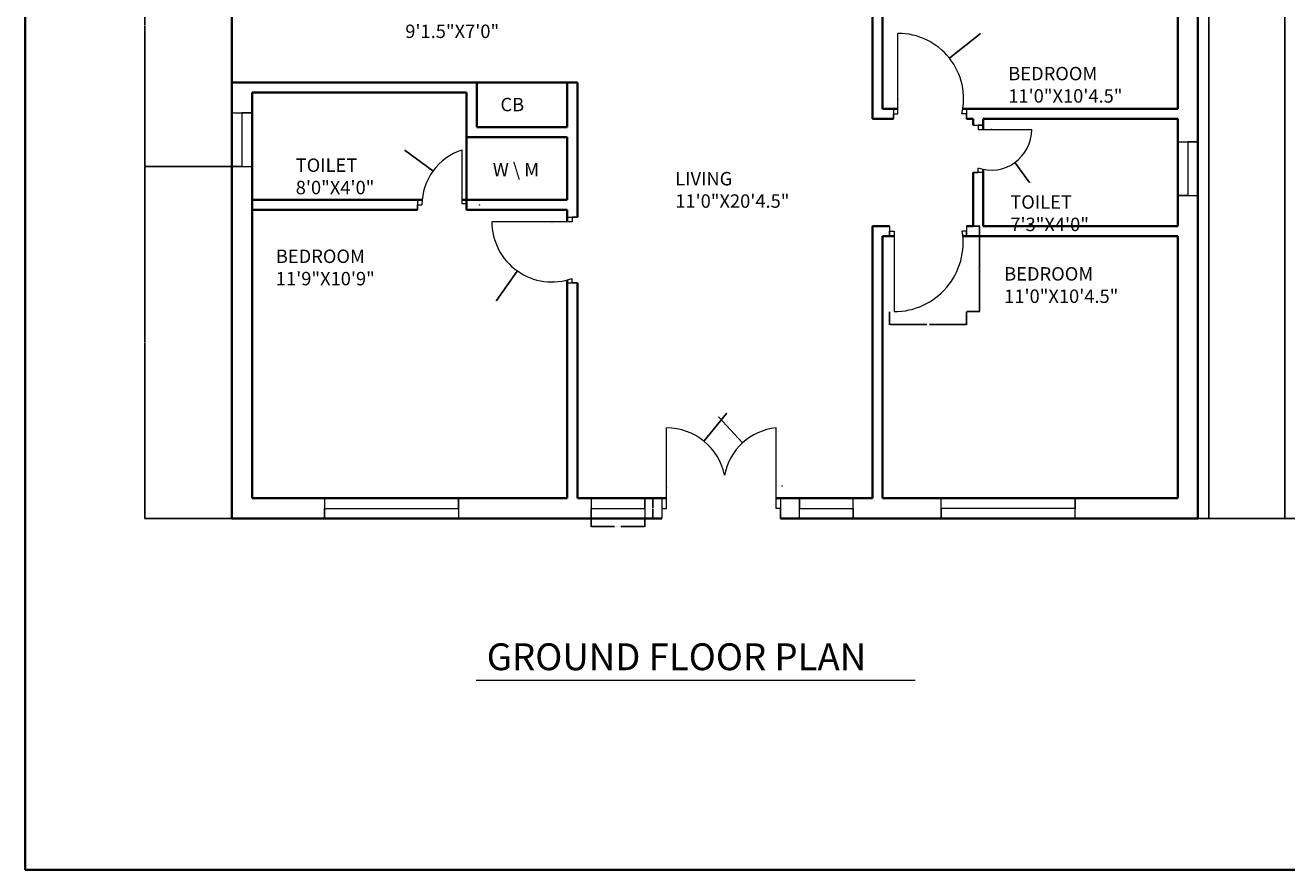
# Model space of a CAD drawing. Units: inches. Extents: x 2250 to 3547, y 1387 to 2604.
# Tile 1 of 11: x 2250 to 2814, y 1387 to 1765. Entities that reach past the tile are written whole.
import ezdxf

# ---------------------------------------------------------------- set-up
doc = ezdxf.new("R2010")
doc.units = ezdxf.units.IN
for name, color, linetype, lineweight in [('A-ANNO-DIMS', 2, 'Continuous', 18), ('A-ANNO-TEXT', 7, 'Continuous', 18), ('A-ANNO-TTLB', 7, 'Continuous', 35), ('A-AREA-IDEN', 7, 'Continuous', 18), ('A-DOOR', 3, 'Continuous', 18), ('A-GLAZ', 4, 'Continuous', 18), ('A-WALL', 7, 'Continuous', 35)]:
    doc.layers.add(name, color=color, linetype=linetype, lineweight=lineweight)
doc.styles.get("Standard").update_dxf_attribs({"font": 'arial.ttf'})
doc.dimstyles.get("Standard").update_dxf_attribs({"dimtxt": 0.18, "dimasz": 0.18, "dimexe": 0.18, "dimexo": 0.0625, "dimgap": 0.09, "dimtad": 0, "dimtih": 1, "dimtoh": 1, "dimdec": 4, "dimzin": 0, "dimdsep": 46, "dimtxsty": 'Standard', "dimcen": 0.09, "dimadec": 0, "dimazin": 0, "dimtfac": 1, "dimtdec": 4, "dimtofl": 0, "dimtmove": 0, "dimatfit": 3, "dimfxl": 1, "dimtolj": 1, "dimtzin": 0, "dimarcsym": 0})

# ---------------------------------------------------------------- blocks, each defined once
blk = doc.blocks.new('WIN-24')
for p, q in [((0, 24), (9, 24)), ((9, 24), (4.5, 24)), ((4.5, 24), (4.5, 0)), ((4.5, 0), (0, 0)), ((0, 0), (9, 0))]:
    blk.add_line(p, q)
blk = doc.blocks.new('WIN-60')
for p, q in [((0, 9), (0, 0)), ((60, 4.5), (60, 9)), ((60, 9), (60, 0)), ((0, 0), (0, 4.5)), ((0, 4.5), (60, 4.5))]:
    blk.add_line(p, q)
blk = doc.blocks.new('WIN-24-SPLIT')
for p, q in [((0, 9), (0, 0)), ((24, 4.5), (24, 9)), ((24, 9), (24, 0)), ((0, 0), (0, 4.5)), ((0, 4.5), (12, 4.5)), ((12, 4.5), (24, 4.5))]:
    blk.add_line(p, q)
blk = doc.blocks.new('DOOR-ENTRY-DOUBLE-SOUTH')
for p, q in [((2, 4.5), (2, 40.5)), ((51.02, 4.5), (51.02, 40.5)), ((0, 9), (0, 0)), ((53.02, 9), (53.02, 0)), ((0, 4.5), (2, 4.5)), ((53.02, 4.5), (51.02, 4.5)), ((53.02, 0), (53.02, 4.5))]:
    blk.add_line(p, q)
for centre, radius, start, end in [((2, 13.91), 26.59, 11.9677, 90), ((53.68, 14.51), 26.13, 95.8256, 169.162)]:
    blk.add_arc(centre, radius, start, end)
blk = doc.blocks.new('DOOR-BED-SOUTHEAST')
for p, q in [((0, 38.25), (0, 33.75)), ((0, 33.75), (0, 36)), ((0, 36), (2, 36)), ((2, 36), (2, 0)), ((34.44, 36), (32.44, 36)), ((34.44, 38.25), (34.44, 33.75)), ((34.44, 33.75), (34.44, 36))]:
    blk.add_line(p, q)
blk.add_arc((2, 30.87), 30.87, 270, 9.5589)
blk = doc.blocks.new('DOOR-BED-WEST-S')
for p, q in [((33.75, 29.39), (38.25, 29.39)), ((38.25, 29.39), (36, 29.39)), ((36, 29.39), (36, 27.39)), ((36, 27.39), (0, 27.39)), ((36, 0), (36, 2)), ((33.75, 0), (38.25, 0)), ((38.25, 0), (36, 0))]:
    blk.add_line(p, q)
blk.add_arc((26.95, 27.39), 26.95, 180, 289.6121)
blk = doc.blocks.new('DOOR-BED-EAST-S')
for p, q in [((2, 2.25), (2, 38.25)), ((0, 4.5), (0, 0)), ((0, 0), (0, 2.25)), ((0, 2.25), (2, 2.25)), ((32.6, 2.25), (30.6, 2.25)), ((32.6, 4.5), (32.6, 0)), ((32.6, 0), (32.6, 2.25))]:
    blk.add_line(p, q)
blk.add_arc((2, 8.89), 29.36, 346.921, 90)
blk = doc.blocks.new('DOOR-BATH-EAST-S')
for p, q in [((0, 21.23), (4.5, 21.23)), ((4.5, 21.23), (2.25, 21.23)), ((2.25, 21.23), (2.25, 19.23)), ((2.25, 19.23), (26.25, 19.23)), ((4.5, 0), (0, 0)), ((0, 0), (2.25, 0)), ((2.25, 0), (2.25, 2))]:
    blk.add_line(p, q)
blk.add_arc((8.07, 19.23), 18.18, 251.336, 0)
blk = doc.blocks.new('DOOR-BATH-WEST-S')
for p, q in [((19.98, 2.81), (19.98, 26.81)), ((0, 4.5), (0, 0)), ((0, 0), (0, 2.25)), ((0, 2.25), (2, 2.25)), ((21.98, 2.81), (19.98, 2.81)), ((21.98, 0), (21.98, 2.81))]:
    blk.add_line(p, q)
blk.add_arc((27.76, 2.25), 25.76, 107.5855, 180)
blk = doc.blocks.new('*D34')
at = {"layer": 'A-ANNO-DIMS', "color": 0, "lineweight": -2, "transparency": 16777216}
for p, q in [((2503.17, 1543.86), (2503.17, 1540.14)), ((2503.35, 1540.32), (2513.67, 1540.32)), ((2526.99, 1540.32), (2516.67, 1540.32)), ((2527.17, 1543.86), (2527.17, 1540.14))]:
    blk.add_line(p, q, dxfattribs=at)
at = {"layer": 'A-ANNO-DIMS', "color": 0, "transparency": 16777216}
for points in [[(2503.35, 1540.35), (2503.35, 1540.29), (2503.17, 1540.32)], [(2526.99, 1540.35), (2526.99, 1540.29), (2527.17, 1540.32)]]:
    blk.add_solid(points, dxfattribs=at)
at = {"layer": 'Defpoints', "color": 0, "transparency": 16777216}
for p in [(2503.17, 1543.92), (2527.17, 1543.92), (2527.17, 1540.32)]:
    blk.add_point(p, dxfattribs=at)
at = {"layer": 'A-ANNO-DIMS', "color": 0, "transparency": 16777216, "insert": (2515.17, 1540.32), "char_height": 0.18, "attachment_point": 5}
blk.add_mtext('\\A1;SPLIT WINDOW 24 TYP.', dxfattribs=at)
blk = doc.blocks.new('*D35')
at = {"layer": 'A-ANNO-DIMS', "color": 0, "lineweight": -2, "transparency": 16777216}
for p, q in [((2527.23, 1552.92), (2530.95, 1552.92)), ((2530.77, 1552.74), (2530.77, 1548.61)), ((2530.77, 1544.1), (2530.77, 1548.24)), ((2527.23, 1543.92), (2530.95, 1543.92))]:
    blk.add_line(p, q, dxfattribs=at)
at = {"layer": 'A-ANNO-DIMS', "color": 0, "transparency": 16777216}
for points in [[(2530.74, 1552.74), (2530.8, 1552.74), (2530.77, 1552.92)], [(2530.74, 1544.1), (2530.8, 1544.1), (2530.77, 1543.92)]]:
    blk.add_solid(points, dxfattribs=at)
at = {"layer": 'Defpoints', "color": 0, "transparency": 16777216}
for p in [(2527.17, 1552.92), (2530.77, 1552.92), (2527.17, 1543.92)]:
    blk.add_point(p, dxfattribs=at)
at = {"layer": 'A-ANNO-DIMS', "color": 0, "transparency": 16777216, "insert": (2530.77, 1548.42), "char_height": 0.18, "attachment_point": 5}
blk.add_mtext('\\A1;9 TYP.', dxfattribs=at)
blk = doc.blocks.new('*D46')
at = {"layer": 'A-ANNO-DIMS', "color": 0, "lineweight": -2, "transparency": 16777216}
for p, q in [((2671.22, 1674.7), (2677.08, 1674.7)), ((2676.9, 1674.52), (2676.9, 1655.75)), ((2676.9, 1636.63), (2676.9, 1655.39)), ((2671.22, 1636.45), (2677.08, 1636.45))]:
    blk.add_line(p, q, dxfattribs=at)
at = {"layer": 'A-ANNO-DIMS', "color": 0, "transparency": 16777216}
for points in [[(2676.87, 1674.52), (2676.93, 1674.52), (2676.9, 1674.7)], [(2676.87, 1636.63), (2676.93, 1636.63), (2676.9, 1636.45)]]:
    blk.add_solid(points, dxfattribs=at)
at = {"layer": 'Defpoints', "color": 0, "transparency": 16777216}
for p in [(2671.16, 1674.7), (2676.9, 1674.7), (2671.16, 1636.45)]:
    blk.add_point(p, dxfattribs=at)
at = {"layer": 'A-ANNO-DIMS', "color": 0, "transparency": 16777216, "insert": (2676.9, 1655.57), "char_height": 0.18, "attachment_point": 5}
blk.add_mtext('\\A1;DOOR 38 TYP.', dxfattribs=at)
blk = doc.blocks.new('*D47')
at = {"layer": 'A-ANNO-DIMS', "color": 0, "lineweight": -2, "transparency": 16777216}
for p, q in [((2636.72, 1636.38), (2636.72, 1630.53)), ((2671.16, 1636.38), (2671.16, 1630.53)), ((2636.9, 1630.71), (2653.41, 1630.71)), ((2670.98, 1630.71), (2654.47, 1630.71))]:
    blk.add_line(p, q, dxfattribs=at)
at = {"layer": 'A-ANNO-DIMS', "color": 0, "transparency": 16777216}
for points in [[(2636.9, 1630.74), (2636.9, 1630.68), (2636.72, 1630.71)], [(2670.98, 1630.74), (2670.98, 1630.68), (2671.16, 1630.71)]]:
    blk.add_solid(points, dxfattribs=at)
at = {"layer": 'Defpoints', "color": 0, "transparency": 16777216}
for p in [(2636.72, 1636.45), (2671.16, 1636.45), (2671.16, 1630.71)]:
    blk.add_point(p, dxfattribs=at)
at = {"layer": 'A-ANNO-DIMS', "color": 0, "transparency": 16777216, "insert": (2653.94, 1630.71), "char_height": 0.18, "attachment_point": 5}
blk.add_mtext('\\A1;34 TYP.', dxfattribs=at)
blk = doc.blocks.new('*D77')
at = {"layer": 'A-ANNO-DIMS', "color": 0, "lineweight": -2, "transparency": 16777216}
for p, q in [((2633.6, 2245.18), (2813.67, 2245.18)), ((2813.49, 2245), (2813.49, 1894.73)), ((2813.49, 1544.1), (2813.49, 1894.37)), ((2774.6, 1543.92), (2813.67, 1543.92))]:
    blk.add_line(p, q, dxfattribs=at)
at = {"layer": 'A-ANNO-DIMS', "color": 0, "transparency": 16777216}
for points in [[(2813.46, 2245), (2813.52, 2245), (2813.49, 2245.18)], [(2813.46, 1544.1), (2813.52, 1544.1), (2813.49, 1543.92)]]:
    blk.add_solid(points, dxfattribs=at)
at = {"layer": 'Defpoints', "color": 0, "transparency": 16777216}
for p in [(2633.54, 2245.18), (2813.49, 2245.18), (2774.54, 1543.92)]:
    blk.add_point(p, dxfattribs=at)
at = {"layer": 'A-ANNO-DIMS', "color": 0, "transparency": 16777216, "insert": (2813.49, 1894.55), "char_height": 0.18, "attachment_point": 5}
blk.add_mtext('\\A1;701.3', dxfattribs=at)
blk = doc.blocks.new('*D78')
at = {"layer": 'A-ANNO-DIMS', "color": 0, "lineweight": -2, "transparency": 16777216}
for p, q in [((2342.48, 1701.32), (2303.41, 1701.32)), ((2303.59, 1701.14), (2303.59, 1622.8)), ((2303.59, 1544.1), (2303.59, 1622.44)), ((2342.48, 1543.92), (2303.41, 1543.92))]:
    blk.add_line(p, q, dxfattribs=at)
at = {"layer": 'A-ANNO-DIMS', "color": 0, "transparency": 16777216}
for points in [[(2303.56, 1701.14), (2303.62, 1701.14), (2303.59, 1701.32)], [(2303.56, 1544.1), (2303.62, 1544.1), (2303.59, 1543.92)]]:
    blk.add_solid(points, dxfattribs=at)
at = {"layer": 'Defpoints', "color": 0, "transparency": 16777216}
for p in [(2303.59, 1701.32), (2342.54, 1701.32), (2342.54, 1543.92)]:
    blk.add_point(p, dxfattribs=at)
at = {"layer": 'A-ANNO-DIMS', "color": 0, "transparency": 16777216, "insert": (2303.59, 1622.62), "char_height": 0.18, "attachment_point": 5}
blk.add_mtext('\\A1;157.4', dxfattribs=at)
blk = doc.blocks.new('*D79')
at = {"layer": 'A-ANNO-DIMS', "color": 0, "lineweight": -2, "transparency": 16777216}
for p, q in [((2342.48, 1827.42), (2303.41, 1827.42)), ((2303.59, 1827.24), (2303.59, 1764.55)), ((2303.59, 1701.5), (2303.59, 1764.19)), ((2342.48, 1701.32), (2303.41, 1701.32))]:
    blk.add_line(p, q, dxfattribs=at)
at = {"layer": 'A-ANNO-DIMS', "color": 0, "transparency": 16777216}
for points in [[(2303.56, 1827.24), (2303.62, 1827.24), (2303.59, 1827.42)], [(2303.56, 1701.5), (2303.62, 1701.5), (2303.59, 1701.32)]]:
    blk.add_solid(points, dxfattribs=at)
at = {"layer": 'Defpoints', "color": 0, "transparency": 16777216}
for p in [(2303.59, 1827.42), (2342.54, 1827.42), (2342.54, 1701.32)]:
    blk.add_point(p, dxfattribs=at)
at = {"layer": 'A-ANNO-DIMS', "color": 0, "transparency": 16777216, "insert": (2303.59, 1764.37), "char_height": 0.18, "attachment_point": 5}
blk.add_mtext('\\A1;126.1', dxfattribs=at)
blk = doc.blocks.new('*D85')
at = {"layer": 'A-ANNO-DIMS', "color": 0, "lineweight": -2, "transparency": 16777216}
for p, q in [((3001.57, 2245.18), (2779.34, 2245.18)), ((2779.52, 2245), (2779.52, 1894.73)), ((2779.52, 1544.1), (2779.52, 1894.37)), ((2851.57, 1543.92), (2779.34, 1543.92))]:
    blk.add_line(p, q, dxfattribs=at)
at = {"layer": 'A-ANNO-DIMS', "color": 0, "transparency": 16777216}
for points in [[(2779.49, 2245), (2779.55, 2245), (2779.52, 2245.18)], [(2779.49, 1544.1), (2779.55, 1544.1), (2779.52, 1543.92)]]:
    blk.add_solid(points, dxfattribs=at)
at = {"layer": 'Defpoints', "color": 0, "transparency": 16777216}
for p in [(2779.52, 2245.18), (3001.63, 2245.18), (2851.63, 1543.92)]:
    blk.add_point(p, dxfattribs=at)
at = {"layer": 'A-ANNO-DIMS', "color": 0, "transparency": 16777216, "insert": (2779.52, 1894.55), "char_height": 0.18, "attachment_point": 5}
blk.add_mtext('\\A1;701.3', dxfattribs=at)
blk = doc.blocks.new('*D118')
at = {"layer": 'A-ANNO-DIMS', "color": 0, "lineweight": -2, "transparency": 16777216}
for p, q in [((2677.22, 1760.8), (2663.57, 1749.96)), ((2677.4, 1760.8), (2677.22, 1760.8)), ((2640.35, 1731.59), (2640.53, 1731.59)), ((2640.44, 1731.5), (2640.44, 1731.68))]:
    blk.add_line(p, q, dxfattribs=at)
at = {"layer": 'A-ANNO-DIMS', "color": 0, "transparency": 16777216}
blk.add_solid([(2663.55, 1749.98), (2663.59, 1749.94), (2663.43, 1749.85)], dxfattribs=at)
at = {"layer": 'Defpoints', "color": 0, "transparency": 16777216}
for p in [(2663.43, 1749.85), (2640.44, 1731.59)]:
    blk.add_point(p, dxfattribs=at)
at = {"layer": 'A-ANNO-DIMS', "color": 0, "transparency": 16777216, "insert": (2677.95, 1760.8), "char_height": 0.18, "attachment_point": 5}
blk.add_mtext('\\A1;R29.357', dxfattribs=at)
blk = doc.blocks.new('*D120')
at = {"layer": 'A-ANNO-DIMS', "color": 0, "lineweight": -2, "transparency": 16777216}
for p, q in [((2485.65, 1676.67), (2485.83, 1676.67)), ((2485.74, 1676.58), (2485.74, 1676.76)), ((2460.89, 1641.43), (2470.1, 1654.5)), ((2460.71, 1641.43), (2460.89, 1641.43))]:
    blk.add_line(p, q, dxfattribs=at)
at = {"layer": 'A-ANNO-DIMS', "color": 0, "transparency": 16777216}
blk.add_solid([(2470.08, 1654.51), (2470.13, 1654.48), (2470.21, 1654.64)], dxfattribs=at)
at = {"layer": 'Defpoints', "color": 0, "transparency": 16777216}
for p in [(2485.74, 1676.67), (2470.21, 1654.64)]:
    blk.add_point(p, dxfattribs=at)
at = {"layer": 'A-ANNO-DIMS', "color": 0, "transparency": 16777216, "insert": (2460.16, 1641.43), "char_height": 0.18, "attachment_point": 5}
blk.add_mtext('\\A1;R26.953', dxfattribs=at)
blk = doc.blocks.new('*D121')
at = {"layer": 'A-ANNO-DIMS', "color": 0, "lineweight": -2, "transparency": 16777216}
for p, q in [((2563.69, 1590.89), (2553.76, 1578.63)), ((2563.87, 1590.89), (2563.69, 1590.89)), ((2536.81, 1557.83), (2536.99, 1557.83)), ((2536.9, 1557.74), (2536.9, 1557.92))]:
    blk.add_line(p, q, dxfattribs=at)
at = {"layer": 'A-ANNO-DIMS', "color": 0, "transparency": 16777216}
blk.add_solid([(2553.73, 1578.65), (2553.78, 1578.61), (2553.64, 1578.49)], dxfattribs=at)
at = {"layer": 'Defpoints', "color": 0, "transparency": 16777216}
for p in [(2553.64, 1578.49), (2536.9, 1557.83)]:
    blk.add_point(p, dxfattribs=at)
at = {"layer": 'A-ANNO-DIMS', "color": 0, "transparency": 16777216, "insert": (2564.42, 1590.89), "char_height": 0.18, "attachment_point": 5}
blk.add_mtext('\\A1;R26.593', dxfattribs=at)
blk = doc.blocks.new('*D123')
at = {"layer": 'A-ANNO-DIMS', "color": 0, "lineweight": -2, "transparency": 16777216}
for p, q in [((2560.16, 1589.26), (2560.34, 1589.26)), ((2560.34, 1589.26), (2570.81, 1577.83)), ((2588.49, 1558.43), (2588.67, 1558.43)), ((2588.58, 1558.34), (2588.58, 1558.52))]:
    blk.add_line(p, q, dxfattribs=at)
at = {"layer": 'A-ANNO-DIMS', "color": 0, "transparency": 16777216}
blk.add_solid([(2570.83, 1577.85), (2570.78, 1577.81), (2570.93, 1577.7)], dxfattribs=at)
at = {"layer": 'Defpoints', "color": 0, "transparency": 16777216}
for p in [(2570.93, 1577.7), (2588.58, 1558.43)]:
    blk.add_point(p, dxfattribs=at)
at = {"layer": 'A-ANNO-DIMS', "color": 0, "transparency": 16777216, "insert": (2559.61, 1589.26), "char_height": 0.18, "attachment_point": 5}
blk.add_mtext('\\A1;R26.126', dxfattribs=at)
blk = doc.blocks.new('*D124')
at = {"layer": 'A-ANNO-DIMS', "color": 0, "lineweight": -2, "transparency": 16777216}
for p, q in [((2419.88, 1708.52), (2420.06, 1708.52)), ((2420.06, 1708.52), (2432.39, 1699.5)), ((2453.23, 1684.17), (2453.41, 1684.17)), ((2453.32, 1684.08), (2453.32, 1684.26))]:
    blk.add_line(p, q, dxfattribs=at)
at = {"layer": 'A-ANNO-DIMS', "color": 0, "transparency": 16777216}
blk.add_solid([(2432.41, 1699.52), (2432.37, 1699.48), (2432.53, 1699.39)], dxfattribs=at)
at = {"layer": 'Defpoints', "color": 0, "transparency": 16777216}
for p in [(2432.53, 1699.39), (2453.32, 1684.17)]:
    blk.add_point(p, dxfattribs=at)
at = {"layer": 'A-ANNO-DIMS', "color": 0, "transparency": 16777216, "insert": (2419.4, 1708.52), "char_height": 0.18, "attachment_point": 5}
blk.add_mtext('\\A1;R25.76', dxfattribs=at)
blk = doc.blocks.new('*D128')
at = {"layer": 'A-ANNO-DIMS', "color": 0, "lineweight": -2, "transparency": 16777216}
for p, q in [((2682.02, 1717.92), (2682.2, 1717.92)), ((2682.11, 1717.83), (2682.11, 1718.01)), ((2699.07, 1694.29), (2692.81, 1703.01)), ((2699.25, 1694.29), (2699.07, 1694.29))]:
    blk.add_line(p, q, dxfattribs=at)
at = {"layer": 'A-ANNO-DIMS', "color": 0, "transparency": 16777216}
blk.add_solid([(2692.84, 1703.02), (2692.79, 1702.99), (2692.71, 1703.15)], dxfattribs=at)
at = {"layer": 'Defpoints', "color": 0, "transparency": 16777216}
for p in [(2682.11, 1717.92), (2692.71, 1703.15)]:
    blk.add_point(p, dxfattribs=at)
at = {"layer": 'A-ANNO-DIMS', "color": 0, "transparency": 16777216, "insert": (2699.73, 1694.29), "char_height": 0.18, "attachment_point": 5}
blk.add_mtext('\\A1;R18.18', dxfattribs=at)

msp = doc.modelspace()

# ---------------------------------------------------------------- linework, layer by layer
at = {"layer": 'A-ANNO-TEXT'}
msp.add_line((2451.7239, 1471.575), (2648.1293, 1471.575), dxfattribs=at)
at = {"layer": 'A-ANNO-TTLB'}
msp.add_lwpolyline([(2250.1093, 2604.1988), (3546.995, 2604.1988), (3546.995, 1386.7251), (2250.1093, 1386.7251)], close=True, dxfattribs=at)
at = {"layer": 'A-WALL'}
for p, q in [((2774.5378, 2232.5639), (2774.5378, 1543.9245)), ((2765.5378, 2037.5639), (2765.5378, 1727.1967)), ((2633.5378, 1856.1967), (2633.5378, 1727.1967)), ((2342.5378, 1827.4245), (2342.5378, 1543.9245)), ((2342.5378, 1827.4245), (2342.5378, 1543.9245)), ((2629.0378, 1818.5639), (2629.0378, 1722.6967)), ((2342.5378, 1738.9245), (2492.5378, 1738.9245)), ((2452.0378, 1719.0224), (2452.0378, 1738.9245)), ((2492.5378, 1738.9245), (2497.0378, 1738.9245)), ((2492.5378, 1738.9245), (2492.5378, 1719.0224)), ((2497.0378, 1738.9245), (2497.0378, 1678.669)), ((2351.5378, 1734.4245), (2447.5378, 1734.4245)), ((2351.5378, 1734.4245), (2351.5378, 1552.9245)), ((2351.5378, 1734.4245), (2351.5378, 1686.4245)), ((2351.5378, 1734.4245), (2447.5378, 1734.4245)), ((2447.5378, 1734.4245), (2447.5378, 1714.5224)), ((2640.439, 1727.1967), (2633.5378, 1727.1967)), ((2765.5378, 1727.1967), (2669.4652, 1727.1967)), ((2633.5378, 1722.6967), (2629.0378, 1722.6967)), ((2638.439, 1722.6967), (2633.5378, 1722.6967)), ((2674.0378, 1722.6967), (2671.0342, 1722.6967)), ((2674.0378, 1722.6967), (2674.0378, 1719.9221)), ((2765.5378, 1722.6967), (2678.5378, 1722.6967)), ((2678.5378, 1717.9221), (2678.5378, 1722.6967)), ((2765.5378, 1722.6967), (2765.5378, 1674.6967)), ((2492.5378, 1719.0224), (2452.0378, 1719.0224)), ((2447.5378, 1714.5224), (2492.5378, 1714.5224)), ((2447.5378, 1714.5224), (2447.5378, 1681.9245)), ((2492.5378, 1714.5224), (2492.5378, 1686.4245)), ((2674.0378, 1698.6967), (2674.0378, 1674.6967)), ((2678.5378, 1674.6967), (2678.5378, 1700.0941)), ((2351.5378, 1686.4245), (2427.6573, 1686.4245)), ((2351.5378, 1681.9245), (2425.5589, 1681.9245)), ((2445.5378, 1686.4245), (2492.5378, 1686.4245)), ((2447.5378, 1681.9245), (2492.5378, 1681.9245)), ((2492.5378, 1681.9245), (2492.5378, 1676.669)), ((2629.0378, 1674.6967), (2636.7154, 1674.6967)), ((2629.0378, 1674.6967), (2629.0378, 1552.9245)), ((2633.5378, 1670.1967), (2633.5378, 1552.9245)), ((2638.7154, 1670.1967), (2633.5378, 1670.1967)), ((2674.0378, 1670.1967), (2669.4542, 1670.1967)), ((2671.1599, 1674.6967), (2674.0378, 1674.6967)), ((2765.5378, 1670.1967), (2674.0378, 1670.1967)), ((2765.5378, 1674.6967), (2678.5378, 1674.6967)), ((2765.5378, 1674.6967), (2678.5378, 1674.6967)), ((2765.5378, 1670.1967), (2765.5378, 1552.9245)), ((2492.5378, 1650.587), (2492.5378, 1552.9245)), ((2497.0378, 1649.2795), (2497.0378, 1552.9245)), ((2351.5378, 1552.9245), (2492.5378, 1552.9245)), ((2497.0378, 1552.9245), (2536.9015, 1552.9245)), ((2585.9248, 1552.9245), (2629.0378, 1552.9245)), ((2633.5378, 1552.9245), (2765.5378, 1552.9245)), ((2342.5378, 1543.9245), (2534.9015, 1543.9245)), ((2587.9248, 1543.9245), (2774.5378, 1543.9245))]:
    msp.add_line(p, q, dxfattribs=at)

# ---------------------------------------------------------------- block references
at = {"layer": 'A-DOOR'}
for name, p in [('DOOR-BED-EAST-S', (2638.439, 1722.6967)), ('DOOR-BATH-EAST-S', (2674.0378, 1698.6967)), ('DOOR-BATH-WEST-S', (2425.5589, 1681.9245)), ('DOOR-BED-WEST-S', (2458.7878, 1649.2795)), ('DOOR-BED-SOUTHEAST', (2636.7154, 1636.4467)), ('DOOR-ENTRY-DOUBLE-SOUTH', (2534.9015, 1543.9245))]:
    msp.add_blockref(name, p, dxfattribs=at)
at = {"layer": 'A-GLAZ'}
for name, p in [('WIN-24', (2342.5378, 1701.3211)), ('WIN-24', (2765.5378, 1688.3924)), ('WIN-60', (2383.9389, 1543.9245)), ('WIN-24-SPLIT', (2503.1695, 1543.9245))]:
    msp.add_blockref(name, p, dxfattribs=at)
for name, p, rotation in [('WIN-24', (2620.3725, 1543.9245), 90.00000000000003), ('WIN-60', (2719.744, 1552.9245), 180)]:
    msp.add_blockref(name, p, dxfattribs=dict(at, rotation=rotation))

# ---------------------------------------------------------------- texts
at = {"layer": 'A-ANNO-TEXT', "insert": (2456.5178, 1488.0269), "char_height": 12, "attachment_point": 1}
msp.add_mtext_dynamic_manual_height_columns('GROUND FLOOR PLAN', width=636.727364, gutter_width=12.5, heights=[0], dxfattribs=at)
at = {"layer": 'A-AREA-IDEN', "char_height": 6, "attachment_point": 1}
for s, width, insert in [('KITCHEN\\P9\'1.5"X7\'0"', 97.961769, (2420.0878, 1774.8651)), ('BEDROOM\\P11\'0"X10\'4.5"', 143.93231, (2689.7696, 1745.9394)), ('CB', 44.566869, (2462.6419, 1732.0874)), ('TOILET\\P8\'0"X4\'0"', 78.851075, (2371.0918, 1704.9523)), ('W \\\\ M', 51.713207, (2459.2085, 1702.9904)), ('LIVING\\P11\'0"X20\'4.5"', 112.323739, (2540.8283, 1698.9136)), ('TOILET\\P7\'3"X4\'0"', 49.508333, (2690.6826, 1688.471)), ('BEDROOM\\P11\'9"X10\'9"', 195.684104, (2362.2, 1664.2126)), ('BEDROOM\\P11\'0"X10\'4.5"', 96.286418, (2687.937, 1656.3352))]:
    msp.add_mtext_dynamic_manual_height_columns(s, width=width, gutter_width=12.5, heights=[0], dxfattribs=dict(at, insert=insert))

# ---------------------------------------------------------------- dimensions: what is measured, and where the dimension line sits
at = {"layer": 'A-ANNO-DIMS'}
for base, p1, p2, picture, middle in [((2813.4878, 2245.1762), (2774.5378, 1543.9245), (2633.5378, 2245.1762), '*D77', (2813.4878, 1894.5504)), ((2779.5165, 2245.1762), (2851.6288, 1543.9245), (3001.6288, 2245.1762), '*D85', (2779.5165, 1894.5504)), ((2303.5878, 1827.4245), (2342.5378, 1701.3211), (2342.5378, 1827.4245), '*D79', (2303.5878, 1764.3728)), ((2303.5878, 1701.3211), (2342.5378, 1543.9245), (2342.5378, 1701.3211), '*D78', (2303.5878, 1622.6228))]:
    dim = msp.add_linear_dim(base=base, p1=p1, p2=p2, angle=90, dimstyle='Standard', override={"dimdec": 1, "dimlfac": 1, "dimrnd": 0, "dimzin": 0, "dimdsep": 46, "dimlunit": 2}, dxfattribs=at)
    dim.commit()
    dim.dimension.update_dxf_attribs({"geometry": picture, "text_midpoint": middle})
for center, mpoint, override, picture, middle in [((2640.439, 1731.5899), (2663.4263, 1749.8492), {"dimdec": 3, "dimlfac": 1, "dimrnd": 0, "dimzin": 0, "dimdsep": 46, "dimlunit": 2}, '*D118', (2677.9484, 1760.8049)), ((2682.1062, 1717.9221), (2692.7078, 1703.1513), {"dimdec": 2, "dimlfac": 1, "dimrnd": 0, "dimzin": 0, "dimdsep": 46, "dimlunit": 2}, '*D128', (2699.7287, 1694.2888)), ((2453.3214, 1684.1745), (2432.5341, 1699.3929), {"dimdec": 2, "dimlfac": 1, "dimrnd": 0, "dimzin": 0, "dimdsep": 46, "dimlunit": 2}, '*D124', (2419.402, 1708.5239)), ((2485.741, 1676.669), (2470.2068, 1654.6427), {"dimdec": 3, "dimlfac": 1, "dimrnd": 0, "dimzin": 0, "dimdsep": 46, "dimlunit": 2}, '*D120', (2460.1565, 1641.4268)), ((2536.9015, 1557.8316), (2553.6432, 1578.4932), {"dimdec": 3, "dimlfac": 1, "dimrnd": 0, "dimzin": 0, "dimdsep": 46, "dimlunit": 2}, '*D121', (2564.4179, 1590.8902)), ((2588.5766, 1558.4333), (2570.9278, 1577.6972), {"dimdec": 3, "dimlfac": 1, "dimrnd": 0, "dimzin": 0, "dimdsep": 46, "dimlunit": 2}, '*D123', (2559.6089, 1589.2555))]:
    dim = msp.add_radius_dim(center=center, mpoint=mpoint, dimstyle='Standard', override=override, dxfattribs=at)
    dim.commit()
    dim.dimension.update_dxf_attribs({"geometry": picture, "text_midpoint": middle, "dimtype": 164})
for base, p1, p2, text, picture, middle in [((2676.8974, 1674.6967), (2671.1599, 1636.4467), (2671.1599, 1674.6967), 'DOOR <> TYP.', '*D46', (2676.8974, 1655.5717)), ((2530.7695, 1552.9245), (2527.1695, 1543.9245), (2527.1695, 1552.9245), '<> TYP.', '*D35', (2530.7695, 1548.4245))]:
    dim = msp.add_linear_dim(base=base, p1=p1, p2=p2, angle=90, text=text, dimstyle='Standard', override={"dimdec": 0, "dimlfac": 1, "dimrnd": 0, "dimzin": 0, "dimdsep": 46, "dimlunit": 2}, dxfattribs=at)
    dim.commit()
    dim.dimension.update_dxf_attribs({"geometry": picture, "text_midpoint": middle})
for base, p1, p2, text, picture, middle in [((2671.1599, 1630.7092), (2636.7154, 1636.4467), (2671.1599, 1636.4467), '<> TYP.', '*D47', (2653.9376, 1630.7092)), ((2527.1695, 1540.3245), (2503.1695, 1543.9245), (2527.1695, 1543.9245), 'SPLIT WINDOW <> TYP.', '*D34', (2515.1695, 1540.3245))]:
    dim = msp.add_linear_dim(base=base, p1=p1, p2=p2, text=text, dimstyle='Standard', override={"dimdec": 0, "dimlfac": 1, "dimrnd": 0, "dimzin": 0, "dimdsep": 46, "dimlunit": 2}, dxfattribs=at)
    dim.commit()
    dim.dimension.update_dxf_attribs({"geometry": picture, "text_midpoint": middle})

doc.saveas('drawing.dxf')
